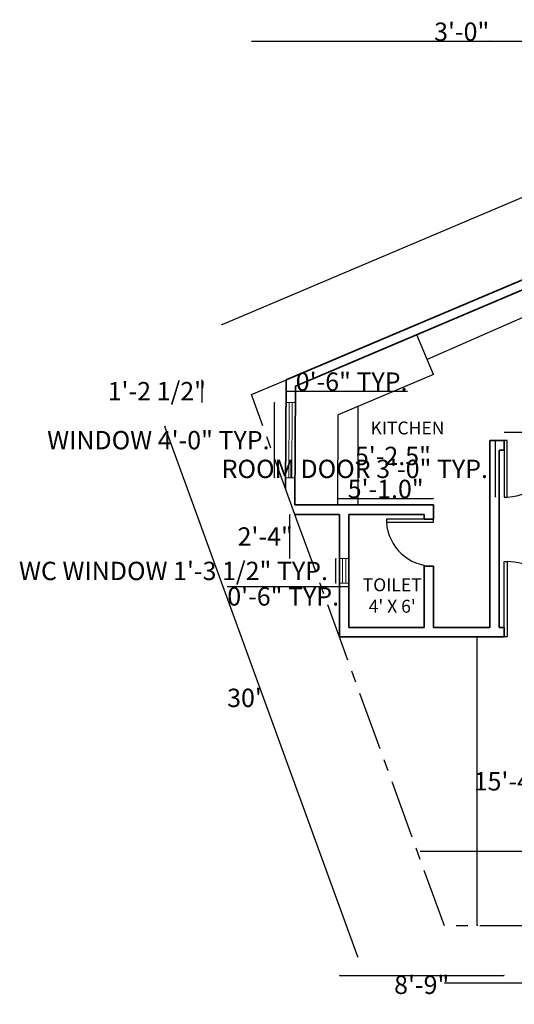
# Model space of a CAD drawing. Units: inches. Extents: x -496 to 183, y 146 to 778.
# Tile 1 of 2: x -496 to -180, y 151 to 778. Entities that reach past the tile are written whole.
import ezdxf

# ---------------------------------------------------------------- set-up
doc = ezdxf.new("R2010")
doc.units = ezdxf.units.IN
doc.header["$MEASUREMENT"] = 0
doc.linetypes.add('CENTER', pattern=[2, 1.25, -0.25, 0.25, -0.25])
for name, color, linetype, lineweight in [('A-ANNO-DIMS', 5, 'Continuous', 18), ('A-AREA-IDEN', 7, 'Continuous', 18), ('A-DOOR', 30, 'Continuous', 25), ('A-FLOR-FIXT', 8, 'Continuous', 25), ('A-GLAZ', 2, 'Continuous', 18), ('A-WALL', 7, 'Continuous', 35), ('C-PROP', 3, 'CENTER', 25)]:
    doc.layers.add(name, color=color, linetype=linetype, lineweight=lineweight)
doc.styles.get("Standard").update_dxf_attribs({"font": 'arial.ttf'})
doc.dimstyles.get("Standard").update_dxf_attribs({"dimtxt": 11.68, "dimasz": 0.18, "dimexe": 0.18, "dimexo": 0.0625, "dimgap": 0.09, "dimtad": 2, "dimtih": 1, "dimtoh": 1, "dimdec": 1, "dimzin": 0, "dimdsep": 46, "dimlunit": 3, "dimtxsty": 'Standard', "dimblk": 'OPEN30', "dimcen": 0.09, "dimse1": 1, "dimse2": 1, "dimadec": 0, "dimazin": 0, "dimtfac": 1, "dimtdec": 1, "dimtofl": 0, "dimtmove": 0, "dimatfit": 3, "dimfxl": 1, "dimtolj": 1, "dimtzin": 0, "dimarcsym": 0})

# ---------------------------------------------------------------- blocks, each defined once
blk = doc.blocks.new('_Open30')
at = {"color": 0, "linetype": 'ByBlock', "lineweight": -2}
for p, q in [((-1, 0.27), (0, 0)), ((0, 0), (-1, -0.27)), ((0, 0), (-1, 0))]:
    blk.add_line(p, q, dxfattribs=at)
blk = doc.blocks.new('*D3')
at = {"layer": 'A-ANNO-DIMS', "color": 0, "lineweight": -2, "ltscale": 5, "transparency": 16777216}
blk.add_line((-224.62, 164.47), (15.02, 164.47), dxfattribs=at)
at = {"layer": 'Defpoints', "color": 0, "ltscale": 5, "transparency": 16777216}
for p in [(-224.8, 200.81), (15.2, 200.81), (15.2, 164.47)]:
    blk.add_point(p, dxfattribs=at)
at = {"layer": 'A-ANNO-DIMS', "color": 0, "lineweight": -2, "ltscale": 5, "transparency": 16777216, "xscale": 0.18, "yscale": 0.18, "zscale": 0.18, "rotation": 180}
blk.add_blockref('_Open30', (-224.8, 164.47), dxfattribs=at)
at = {"layer": 'A-ANNO-DIMS', "color": 0, "lineweight": -2, "ltscale": 5, "transparency": 16777216, "xscale": 0.18, "yscale": 0.18, "zscale": 0.18}
blk.add_blockref('_Open30', (15.2, 164.47), dxfattribs=at)
at = {"layer": 'A-ANNO-DIMS', "color": 0, "ltscale": 5, "transparency": 16777216, "insert": (-104.8, 158.42), "char_height": 11.68, "attachment_point": 5}
blk.add_mtext("\\A1;20'", dxfattribs=at)
blk = doc.blocks.new('*D5')
at = {"layer": 'A-ANNO-DIMS', "color": 0, "lineweight": -2, "ltscale": 5, "transparency": 16777216}
blk.add_line((-280.02, 180.9), (-403.03, 518.85), dxfattribs=at)
at = {"layer": 'Defpoints', "color": 0, "ltscale": 5, "transparency": 16777216}
for p in [(-347.92, 539.1), (-403.09, 519.02), (-224.8, 200.81)]:
    blk.add_point(p, dxfattribs=at)
at = {"layer": 'A-ANNO-DIMS', "color": 0, "lineweight": -2, "ltscale": 5, "transparency": 16777216, "xscale": 0.18, "yscale": 0.18, "zscale": 0.18}
for p, rotation in [((-403.09, 519.02), 109.9999999999999), ((-279.96, 180.73), 290)]:
    blk.add_blockref('_Open30', p, dxfattribs=dict(at, rotation=rotation))
at = {"layer": 'A-ANNO-DIMS', "color": 0, "ltscale": 5, "transparency": 16777216, "insert": (-352.3, 345.96), "char_height": 11.68, "attachment_point": 5}
blk.add_mtext("\\A1;30'", dxfattribs=at)
blk = doc.blocks.new('*D6')
at = {"layer": 'A-ANNO-DIMS', "color": 0, "lineweight": -2, "ltscale": 5, "transparency": 16777216}
blk.add_line((-366.62, 583.72), (89.94, 777.08), dxfattribs=at)
at = {"layer": 'Defpoints', "color": 0, "ltscale": 5, "transparency": 16777216}
for p in [(90.11, 777.15), (108.97, 732.61), (-347.92, 539.1)]:
    blk.add_point(p, dxfattribs=at)
at = {"layer": 'A-ANNO-DIMS', "color": 0, "lineweight": -2, "ltscale": 5, "transparency": 16777216, "xscale": 0.18, "yscale": 0.18, "zscale": 0.18}
for p, rotation in [((90.11, 777.15), 22.95381137769926), ((-366.79, 583.64), 202.9538113776993)]:
    blk.add_blockref('_Open30', p, dxfattribs=dict(at, rotation=rotation))
at = {"layer": 'A-ANNO-DIMS', "color": 0, "ltscale": 5, "transparency": 16777216, "insert": (-144.61, 695.21), "char_height": 11.68, "attachment_point": 5}
blk.add_mtext('\\A1;41\'-4.2"', dxfattribs=at)
blk = doc.blocks.new('*D7')
at = {"layer": 'A-ANNO-DIMS', "color": 0, "lineweight": -2, "ltscale": 5, "transparency": 16777216}
blk.add_line((-235.59, 561.64), (-68.58, 635.31), dxfattribs=at)
at = {"layer": 'Defpoints', "color": 0, "ltscale": 5, "transparency": 16777216}
for p in [(-69.77, 638.45), (-68.41, 635.38), (-237.11, 564.64)]:
    blk.add_point(p, dxfattribs=at)
at = {"layer": 'A-ANNO-DIMS', "color": 0, "lineweight": -2, "ltscale": 5, "transparency": 16777216, "xscale": 0.18, "yscale": 0.18, "zscale": 0.18}
for p, rotation in [((-68.41, 635.38), 23.80147962325558), ((-235.75, 561.57), 203.8014796232556)]:
    blk.add_blockref('_Open30', p, dxfattribs=dict(at, rotation=rotation))
at = {"layer": 'A-ANNO-DIMS', "color": 0, "ltscale": 5, "transparency": 16777216, "insert": (-145.55, 583.66), "char_height": 11.68, "attachment_point": 5}
blk.add_mtext('\\A1;15\'-2.9"', dxfattribs=at)
blk = doc.blocks.new('*D12')
at = {"layer": 'A-ANNO-DIMS', "color": 0, "lineweight": -2, "ltscale": 5, "transparency": 16777216}
blk.add_line((22.65, 248.06), (-240.18, 248.06), dxfattribs=at)
at = {"layer": 'Defpoints', "color": 0, "ltscale": 5, "transparency": 16777216}
for p in [(-240.36, 248.06), (-240.36, 243.58), (22.83, 244.08)]:
    blk.add_point(p, dxfattribs=at)
at = {"layer": 'A-ANNO-DIMS', "color": 0, "lineweight": -2, "ltscale": 5, "transparency": 16777216, "xscale": 0.18, "yscale": 0.18, "zscale": 0.18, "rotation": 180}
blk.add_blockref('_Open30', (-240.36, 248.06), dxfattribs=at)
at = {"layer": 'A-ANNO-DIMS', "color": 0, "lineweight": -2, "ltscale": 5, "transparency": 16777216, "xscale": 0.18, "yscale": 0.18, "zscale": 0.18}
blk.add_blockref('_Open30', (22.83, 248.06), dxfattribs=at)
at = {"layer": 'A-ANNO-DIMS', "color": 0, "ltscale": 5, "transparency": 16777216, "insert": (-108.76, 254.01), "char_height": 11.68, "attachment_point": 5}
blk.add_mtext('\\A1;21\'-11.2"', dxfattribs=at)
blk = doc.blocks.new('*D13')
at = {"layer": 'A-ANNO-DIMS', "color": 0, "lineweight": -2, "ltscale": 5, "transparency": 16777216}
blk.add_line((-203.87, 200.99), (-203.87, 384.63), dxfattribs=at)
at = {"layer": 'Defpoints', "color": 0, "ltscale": 5, "transparency": 16777216}
for p in [(-208.53, 384.81), (-203.87, 384.81), (-208.53, 200.81)]:
    blk.add_point(p, dxfattribs=at)
at = {"layer": 'A-ANNO-DIMS', "color": 0, "lineweight": -2, "ltscale": 5, "transparency": 16777216, "xscale": 0.18, "yscale": 0.18, "zscale": 0.18}
for p, rotation in [((-203.87, 384.81), 90), ((-203.87, 200.81), 270)]:
    blk.add_blockref('_Open30', p, dxfattribs=dict(at, rotation=rotation))
at = {"layer": 'A-ANNO-DIMS', "color": 0, "ltscale": 5, "transparency": 16777216, "insert": (-177.47, 292.81), "char_height": 11.68, "attachment_point": 5}
blk.add_mtext('\\A1;15\'-4.0"', dxfattribs=at)
blk = doc.blocks.new('*D14')
at = {"layer": 'A-ANNO-DIMS', "color": 0, "lineweight": -2, "ltscale": 5, "transparency": 16777216}
blk.add_line((-280.06, 531.08), (-280.06, 468.99), dxfattribs=at)
at = {"layer": 'Defpoints', "color": 0, "ltscale": 5, "transparency": 16777216}
for p in [(-280.79, 531.26), (-280.79, 468.81), (-280.06, 468.81)]:
    blk.add_point(p, dxfattribs=at)
at = {"layer": 'A-ANNO-DIMS', "color": 0, "lineweight": -2, "ltscale": 5, "transparency": 16777216, "xscale": 0.18, "yscale": 0.18, "zscale": 0.18}
for p, rotation in [((-280.06, 531.26), 90), ((-280.06, 468.81), 270)]:
    blk.add_blockref('_Open30', p, dxfattribs=dict(at, rotation=rotation))
at = {"layer": 'A-ANNO-DIMS', "color": 0, "ltscale": 5, "transparency": 16777216, "insert": (-257.64, 500.04), "char_height": 11.68, "attachment_point": 5}
blk.add_mtext('\\A1;5\'-2.5"', dxfattribs=at)
blk = doc.blocks.new('*D15')
at = {"layer": 'A-ANNO-DIMS', "color": 0, "lineweight": -2, "ltscale": 5, "transparency": 16777216}
blk.add_line((-292.55, 472.99), (-231.95, 472.99), dxfattribs=at)
at = {"layer": 'Defpoints', "color": 0, "ltscale": 5, "transparency": 16777216}
for p in [(-231.77, 472.99), (-292.73, 468.81), (-231.77, 468.81)]:
    blk.add_point(p, dxfattribs=at)
at = {"layer": 'A-ANNO-DIMS', "color": 0, "lineweight": -2, "ltscale": 5, "transparency": 16777216, "xscale": 0.18, "yscale": 0.18, "zscale": 0.18, "rotation": 180}
blk.add_blockref('_Open30', (-292.73, 472.99), dxfattribs=at)
at = {"layer": 'A-ANNO-DIMS', "color": 0, "lineweight": -2, "ltscale": 5, "transparency": 16777216, "xscale": 0.18, "yscale": 0.18, "zscale": 0.18}
blk.add_blockref('_Open30', (-231.77, 472.99), dxfattribs=at)
at = {"layer": 'A-ANNO-DIMS', "color": 0, "ltscale": 5, "transparency": 16777216, "insert": (-262.25, 479.04), "char_height": 11.68, "attachment_point": 5}
blk.add_mtext('\\A1;5\'-1.0"', dxfattribs=at)
blk = doc.blocks.new('DOOR-SWING-36IN')
at = {"ltscale": 5}
for p, q in [((0, 0), (0, -36)), ((2, 0), (0, 0)), ((2, -36), (2, 0)), ((0, -36), (2, -36))]:
    blk.add_line(p, q, dxfattribs=at)
blk.add_arc((-0.06, 0), 36.06, 273.27315, 0, dxfattribs=at)
blk = doc.blocks.new('DOOR-SWING-30IN')
at = {"ltscale": 5}
for p, q in [((0, 0), (-30, 0)), ((-30, 0), (-30, -2)), ((0, -2), (0, 0)), ((-30, -2), (0, -2))]:
    blk.add_line(p, q, dxfattribs=at)
blk.add_arc((0, 0.07), 30.07, 183.94987, 270, dxfattribs=at)
blk = doc.blocks.new('WIN-48IN')
at = {"ltscale": 5}
for p, q in [((0, 0), (-0.22, -48)), ((0, 0), (6, -0.03)), ((6, -0.03), (5.78, -48.03)), ((-0.22, -48), (5.78, -48.03))]:
    blk.add_line(p, q, dxfattribs=at)
for p, q in [((1.78, -48.01), (2, -0.01)), ((3.78, -48.02), (4, -0.02))]:
    blk.add_line(p, q)
blk = doc.blocks.new('WIN-SMALL-WC')
at = {"ltscale": 5}
for p, q in [((-15.66, -6), (-15.66, 0)), ((-15.66, 0), (0, 0)), ((0, 0), (0, -6)), ((-15.66, -2), (0, -2)), ((0, -4), (-15.66, -4)), ((0, -6), (-15.66, -6))]:
    blk.add_line(p, q, dxfattribs=at)
blk = doc.blocks.new('*D20')
at = {"layer": 'A-ANNO-DIMS', "color": 0, "lineweight": -2, "ltscale": 5, "transparency": 16777216}
blk.add_line((-192.17, 473.99), (-192.17, 509.63), dxfattribs=at)
at = {"layer": 'Defpoints', "color": 0, "ltscale": 5, "transparency": 16777216}
for p in [(-192.17, 509.81), (-186.77, 509.81), (-186.77, 473.81)]:
    blk.add_point(p, dxfattribs=at)
at = {"layer": 'A-ANNO-DIMS', "color": 0, "lineweight": -2, "ltscale": 5, "transparency": 16777216, "xscale": 0.18, "yscale": 0.18, "zscale": 0.18}
for p, rotation in [((-192.17, 509.81), 90), ((-192.17, 473.81), 270)]:
    blk.add_blockref('_Open30', p, dxfattribs=dict(at, rotation=rotation))
at = {"layer": 'A-ANNO-DIMS', "color": 0, "ltscale": 5, "transparency": 16777216, "insert": (-281.94, 491.81), "char_height": 11.68, "attachment_point": 5}
blk.add_mtext('\\A1;ROOM DOOR 3\'-0" TYP.', dxfattribs=at)
blk = doc.blocks.new('*D21')
at = {"layer": 'A-ANNO-DIMS', "color": 0, "lineweight": -2, "ltscale": 5, "transparency": 16777216}
for p, q in [((-186.59, 515.21), (-150.95, 515.21)), ((-150.77, 515.21), (-79.22, 515.21))]:
    blk.add_line(p, q, dxfattribs=at)
at = {"layer": 'Defpoints', "color": 0, "ltscale": 5, "transparency": 16777216}
for p in [(-150.77, 515.21), (-186.77, 509.81), (-150.77, 509.81)]:
    blk.add_point(p, dxfattribs=at)
at = {"layer": 'A-ANNO-DIMS', "color": 0, "lineweight": -2, "ltscale": 5, "transparency": 16777216, "xscale": 0.18, "yscale": 0.18, "zscale": 0.18, "rotation": 180}
blk.add_blockref('_Open30', (-186.77, 515.21), dxfattribs=at)
at = {"layer": 'A-ANNO-DIMS', "color": 0, "lineweight": -2, "ltscale": 5, "transparency": 16777216, "xscale": 0.18, "yscale": 0.18, "zscale": 0.18}
blk.add_blockref('_Open30', (-150.77, 515.21), dxfattribs=at)
at = {"layer": 'A-ANNO-DIMS', "color": 0, "ltscale": 5, "transparency": 16777216, "insert": (-114.9, 521.27), "char_height": 11.68, "attachment_point": 5}
blk.add_mtext('\\A1;3\'-0" TYP.', dxfattribs=at)
blk = doc.blocks.new('*D24')
at = {"layer": 'A-ANNO-DIMS', "color": 0, "lineweight": -2, "ltscale": 5, "transparency": 16777216}
blk.add_line((-333.25, 486.28), (-333.25, 533.95), dxfattribs=at)
at = {"layer": 'Defpoints', "color": 0, "ltscale": 5, "transparency": 16777216}
for p in [(-333.25, 534.13), (-326.05, 534.13), (-326.05, 486.1)]:
    blk.add_point(p, dxfattribs=at)
at = {"layer": 'A-ANNO-DIMS', "color": 0, "lineweight": -2, "ltscale": 5, "transparency": 16777216, "xscale": 0.18, "yscale": 0.18, "zscale": 0.18}
for p, rotation in [((-333.25, 534.13), 90), ((-333.25, 486.1), 270)]:
    blk.add_blockref('_Open30', p, dxfattribs=dict(at, rotation=rotation))
at = {"layer": 'A-ANNO-DIMS', "color": 0, "ltscale": 5, "transparency": 16777216, "insert": (-407.24, 510.11), "char_height": 11.68, "attachment_point": 5}
blk.add_mtext('\\A1;WINDOW 4\'-0" TYP.', dxfattribs=at)
blk = doc.blocks.new('*D25')
at = {"layer": 'A-ANNO-DIMS', "color": 0, "lineweight": -2, "ltscale": 5, "transparency": 16777216}
for p, q in [((-325.87, 541.33), (-320.01, 541.33)), ((-319.83, 541.33), (-248.28, 541.33))]:
    blk.add_line(p, q, dxfattribs=at)
at = {"layer": 'Defpoints', "color": 0, "ltscale": 5, "transparency": 16777216}
for p in [(-319.83, 541.33), (-326.05, 534.13), (-319.83, 534.13)]:
    blk.add_point(p, dxfattribs=at)
at = {"layer": 'A-ANNO-DIMS', "color": 0, "lineweight": -2, "ltscale": 5, "transparency": 16777216, "xscale": 0.18, "yscale": 0.18, "zscale": 0.18, "rotation": 180}
blk.add_blockref('_Open30', (-326.05, 541.33), dxfattribs=at)
at = {"layer": 'A-ANNO-DIMS', "color": 0, "lineweight": -2, "ltscale": 5, "transparency": 16777216, "xscale": 0.18, "yscale": 0.18, "zscale": 0.18}
blk.add_blockref('_Open30', (-319.83, 541.33), dxfattribs=at)
at = {"layer": 'A-ANNO-DIMS', "color": 0, "ltscale": 5, "transparency": 16777216, "insert": (-283.97, 547.38), "char_height": 11.68, "attachment_point": 5}
blk.add_mtext('\\A1;0\'-6" TYP.', dxfattribs=at)
blk = doc.blocks.new('*D26')
at = {"layer": 'A-ANNO-DIMS', "color": 0, "lineweight": -2, "ltscale": 5, "transparency": 16777216}
blk.add_line((-294.11, 419.16), (-294.11, 434.46), dxfattribs=at)
at = {"layer": 'Defpoints', "color": 0, "ltscale": 5, "transparency": 16777216}
for p in [(-294.11, 434.64), (-291.77, 434.64), (-291.77, 418.98)]:
    blk.add_point(p, dxfattribs=at)
at = {"layer": 'A-ANNO-DIMS', "color": 0, "lineweight": -2, "ltscale": 5, "transparency": 16777216, "xscale": 0.18, "yscale": 0.18, "zscale": 0.18}
for p, rotation in [((-294.11, 434.64), 90), ((-294.11, 418.98), 270)]:
    blk.add_blockref('_Open30', p, dxfattribs=dict(at, rotation=rotation))
at = {"layer": 'A-ANNO-DIMS', "color": 0, "ltscale": 5, "transparency": 16777216, "insert": (-397.57, 426.81), "char_height": 11.68, "attachment_point": 5}
blk.add_mtext('\\A1;WC WINDOW 1\'-3 1/2" TYP.', dxfattribs=at)
blk = doc.blocks.new('*D27')
at = {"layer": 'A-ANNO-DIMS', "color": 0, "lineweight": -2, "ltscale": 5, "transparency": 16777216}
for p, q in [((-291.77, 416.64), (-363.32, 416.64)), ((-285.95, 416.64), (-291.59, 416.64))]:
    blk.add_line(p, q, dxfattribs=at)
at = {"layer": 'Defpoints', "color": 0, "ltscale": 5, "transparency": 16777216}
for p in [(-291.77, 418.98), (-291.77, 416.64), (-285.77, 418.98)]:
    blk.add_point(p, dxfattribs=at)
at = {"layer": 'A-ANNO-DIMS', "color": 0, "lineweight": -2, "ltscale": 5, "transparency": 16777216, "xscale": 0.18, "yscale": 0.18, "zscale": 0.18}
for p, rotation in [((-291.77, 416.64), 179.9999999999984), ((-285.77, 416.64), 359.9999999999984)]:
    blk.add_blockref('_Open30', p, dxfattribs=dict(at, rotation=rotation))
at = {"layer": 'A-ANNO-DIMS', "color": 0, "ltscale": 5, "transparency": 16777216, "insert": (-327.63, 410.58), "char_height": 11.68, "attachment_point": 5}
blk.add_mtext('\\A1;0\'-6" TYP.', dxfattribs=at)
blk = doc.blocks.new('*D28')
at = {"layer": 'A-ANNO-DIMS', "color": 0, "lineweight": -2, "ltscale": 5, "transparency": 16777216}
blk.add_line((-347.74, 764.21), (108.79, 764.21), dxfattribs=at)
at = {"layer": 'Defpoints', "color": 0, "ltscale": 5, "transparency": 16777216}
for p in [(108.97, 764.21), (108.97, 732.61), (-347.92, 539.1)]:
    blk.add_point(p, dxfattribs=at)
at = {"layer": 'A-ANNO-DIMS', "color": 0, "lineweight": -2, "ltscale": 5, "transparency": 16777216, "xscale": 0.18, "yscale": 0.18, "zscale": 0.18, "rotation": 180}
blk.add_blockref('_Open30', (-347.92, 764.21), dxfattribs=at)
at = {"layer": 'A-ANNO-DIMS', "color": 0, "lineweight": -2, "ltscale": 5, "transparency": 16777216, "xscale": 0.18, "yscale": 0.18, "zscale": 0.18}
blk.add_blockref('_Open30', (108.97, 764.21), dxfattribs=at)
at = {"layer": 'A-ANNO-DIMS', "color": 0, "ltscale": 5, "transparency": 16777216, "insert": (-119.47, 770.27), "char_height": 11.68, "attachment_point": 5}
blk.add_mtext('\\A1;38\'-1"', dxfattribs=at)
blk = doc.blocks.new('*D31')
at = {"layer": 'A-ANNO-DIMS', "color": 0, "lineweight": -2, "ltscale": 5, "transparency": 16777216}
blk.add_line((-231.59, 764.21), (-195.95, 764.21), dxfattribs=at)
at = {"layer": 'Defpoints', "color": 0, "ltscale": 5, "transparency": 16777216}
for p in [(-195.77, 764.21), (-231.77, 390.81), (-195.77, 390.81)]:
    blk.add_point(p, dxfattribs=at)
at = {"layer": 'A-ANNO-DIMS', "color": 0, "lineweight": -2, "ltscale": 5, "transparency": 16777216, "xscale": 0.18, "yscale": 0.18, "zscale": 0.18, "rotation": 180}
blk.add_blockref('_Open30', (-231.77, 764.21), dxfattribs=at)
at = {"layer": 'A-ANNO-DIMS', "color": 0, "lineweight": -2, "ltscale": 5, "transparency": 16777216, "xscale": 0.18, "yscale": 0.18, "zscale": 0.18}
blk.add_blockref('_Open30', (-195.77, 764.21), dxfattribs=at)
at = {"layer": 'A-ANNO-DIMS', "color": 0, "ltscale": 5, "transparency": 16777216, "insert": (-213.77, 770.27), "char_height": 11.68, "attachment_point": 5}
blk.add_mtext('\\A1;3\'-0"', dxfattribs=at)
blk = doc.blocks.new('*D32')
at = {"layer": 'A-ANNO-DIMS', "color": 0, "lineweight": -2, "ltscale": 5, "transparency": 16777216}
blk.add_line((-291.59, 169.21), (-186.95, 169.21), dxfattribs=at)
at = {"layer": 'Defpoints', "color": 0, "ltscale": 5, "transparency": 16777216}
for p in [(-291.77, 384.81), (-186.77, 384.81), (-186.77, 169.21)]:
    blk.add_point(p, dxfattribs=at)
at = {"layer": 'A-ANNO-DIMS', "color": 0, "lineweight": -2, "ltscale": 5, "transparency": 16777216, "xscale": 0.18, "yscale": 0.18, "zscale": 0.18, "rotation": 180}
blk.add_blockref('_Open30', (-291.77, 169.21), dxfattribs=at)
at = {"layer": 'A-ANNO-DIMS', "color": 0, "lineweight": -2, "ltscale": 5, "transparency": 16777216, "xscale": 0.18, "yscale": 0.18, "zscale": 0.18}
blk.add_blockref('_Open30', (-186.77, 169.21), dxfattribs=at)
at = {"layer": 'A-ANNO-DIMS', "color": 0, "ltscale": 5, "transparency": 16777216, "insert": (-239.27, 163.16), "char_height": 11.68, "attachment_point": 5}
blk.add_mtext('\\A1;8\'-9"', dxfattribs=at)
blk = doc.blocks.new('*D35')
at = {"layer": 'A-ANNO-DIMS', "color": 0, "lineweight": -2, "ltscale": 5, "transparency": 16777216}
blk.add_line((-379.52, 548.3), (-379.52, 534.31), dxfattribs=at)
at = {"layer": 'Defpoints', "color": 0, "ltscale": 5, "transparency": 16777216}
for p in [(-325.77, 548.48), (-379.52, 534.13), (-325.83, 534.13)]:
    blk.add_point(p, dxfattribs=at)
at = {"layer": 'A-ANNO-DIMS', "color": 0, "lineweight": -2, "ltscale": 5, "transparency": 16777216, "xscale": 0.18, "yscale": 0.18, "zscale": 0.18}
for p, rotation in [((-379.52, 548.48), 90), ((-379.52, 534.13), 270)]:
    blk.add_blockref('_Open30', p, dxfattribs=dict(at, rotation=rotation))
at = {"layer": 'A-ANNO-DIMS', "color": 0, "ltscale": 5, "transparency": 16777216, "insert": (-408.2, 541.3), "char_height": 11.68, "attachment_point": 5}
blk.add_mtext('\\A1;1\'-2 1/2"', dxfattribs=at)
blk = doc.blocks.new('*D39')
at = {"layer": 'A-ANNO-DIMS', "color": 0, "lineweight": -2, "ltscale": 5, "transparency": 16777216}
blk.add_line((-323.37, 434.82), (-323.37, 462.63), dxfattribs=at)
at = {"layer": 'Defpoints', "color": 0, "ltscale": 5, "transparency": 16777216}
for p in [(-323.37, 462.81), (-291.77, 462.81), (-291.77, 434.64)]:
    blk.add_point(p, dxfattribs=at)
at = {"layer": 'A-ANNO-DIMS', "color": 0, "lineweight": -2, "ltscale": 5, "transparency": 16777216, "xscale": 0.18, "yscale": 0.18, "zscale": 0.18}
for p, rotation in [((-323.37, 462.81), 90), ((-323.37, 434.64), 270)]:
    blk.add_blockref('_Open30', p, dxfattribs=dict(at, rotation=rotation))
at = {"layer": 'A-ANNO-DIMS', "color": 0, "ltscale": 5, "transparency": 16777216, "insert": (-339.08, 448.73), "char_height": 11.68, "attachment_point": 5}
blk.add_mtext('\\A1;2\'-4"', dxfattribs=at)
blk = doc.blocks.new('*D40')
at = {"layer": 'A-ANNO-DIMS', "color": 0, "lineweight": -2, "ltscale": 5, "transparency": 16777216}
for p, q in [((-131.31, 438), (-151.99, 418.18)), ((-88.99, 438), (-131.31, 438)), ((-186.9, 384.81), (-186.72, 384.81)), ((-186.81, 384.72), (-186.81, 384.9))]:
    blk.add_line(p, q, dxfattribs=at)
at = {"layer": 'Defpoints', "color": 0, "ltscale": 5, "transparency": 16777216}
for p in [(-152.12, 418.05), (-186.81, 384.81)]:
    blk.add_point(p, dxfattribs=at)
at = {"layer": 'A-ANNO-DIMS', "color": 0, "lineweight": -2, "ltscale": 5, "transparency": 16777216, "xscale": 0.18, "yscale": 0.18, "zscale": 0.18, "rotation": 223.7807826130634}
blk.add_blockref('_Open30', (-152.12, 418.05), dxfattribs=at)
at = {"layer": 'A-ANNO-DIMS', "color": 0, "ltscale": 5, "transparency": 16777216, "insert": (-110.11, 444.05), "char_height": 11.68, "attachment_point": 5}
blk.add_mtext('\\A1;R4\'-0"', dxfattribs=at)

msp = doc.modelspace()

# ---------------------------------------------------------------- linework, layer by layer
at = {"layer": 'A-DOOR', "ltscale": 5}
for p, q in [((-186.77, 384.81), (-186.77, 432.81)), ((-186.77, 432.81), (-184.77, 432.81)), ((-184.77, 432.81), (-184.77, 384.81)), ((-184.77, 384.81), (-186.77, 384.81))]:
    msp.add_line(p, q, dxfattribs=at)
msp.add_arc((-186.81, 384.81), 48.04, 0, 87.56225, dxfattribs=at)
at = {"layer": 'A-FLOR-FIXT'}
for p, q in [((-231.77, 552.02), (-242.45, 577.26)), ((-231.77, 552.02), (-292.47, 526.32)), ((-292.73, 468.69), (-292.47, 526.32))]:
    msp.add_line(p, q, dxfattribs=at)
at = {"layer": 'A-WALL', "ltscale": 5}
msp.add_line((-64.98, 658.93), (-325.77, 548.48), dxfattribs=at)
at = {"layer": 'A-WALL'}
for p, q in [((-69.77, 650.39), (-319.79, 544.5)), ((-326.08, 479.1), (-325.77, 548.48)), ((-320.13, 468.81), (-319.79, 544.5)), ((-195.77, 509.81), (-186.77, 509.81)), ((-195.77, 390.81), (-195.77, 509.81)), ((-186.77, 503.81), (-186.77, 509.81)), ((-189.77, 503.81), (-186.77, 503.81)), ((-189.77, 390.81), (-189.77, 503.81)), ((-320.13, 468.81), (-231.77, 468.81)), ((-231.77, 459.81), (-231.77, 468.81)), ((-320.16, 462.81), (-291.77, 462.81)), ((-291.77, 384.81), (-291.77, 462.81)), ((-285.77, 390.81), (-285.77, 462.81)), ((-285.77, 462.81), (-237.77, 462.81)), ((-237.77, 459.81), (-237.77, 462.81)), ((-237.77, 459.81), (-231.77, 459.81)), ((-237.77, 390.81), (-237.77, 429.81)), ((-237.77, 429.81), (-231.77, 429.81)), ((-231.77, 390.81), (-231.77, 429.81)), ((-285.77, 390.81), (-237.77, 390.81)), ((-231.77, 390.81), (-195.77, 390.81)), ((-189.77, 390.81), (-186.77, 390.81)), ((-186.77, 384.81), (-186.77, 390.81)), ((-291.77, 384.81), (-186.77, 384.81))]:
    msp.add_line(p, q, dxfattribs=at)
at = {"layer": 'C-PROP', "ltscale": 30}
msp.add_lwpolyline([(-320.16, 462.81), (-347.92, 539.1), (108.97, 732.61), (15.2, 200.81), (-224.8, 200.81), (-319.06, 459.81)], close=True, dxfattribs=at)

# ---------------------------------------------------------------- block references
at = {"layer": 'A-DOOR'}
for name, p in [('DOOR-SWING-36IN', (-186.77, 509.81)), ('DOOR-SWING-30IN', (-231.77, 459.81))]:
    msp.add_blockref(name, p, dxfattribs=at)
at = {"layer": 'A-GLAZ'}
msp.add_blockref('WIN-48IN', (-325.83, 534.13), dxfattribs=at)
at = {"layer": 'A-GLAZ', "rotation": 89.9999999999982}
msp.add_blockref('WIN-SMALL-WC', (-291.77, 434.64), dxfattribs=at)

# ---------------------------------------------------------------- texts
at = {"layer": 'A-AREA-IDEN', "ltscale": 5, "char_height": 8.2, "attachment_point": 1}
for s, width, insert in [('KITCHEN', 1.3024, (-271.95, 521.96)), ("\\pxqc;TOILET\\P4' X 6'", 37.7679, (-276.97, 422.07))]:
    msp.add_mtext_dynamic_manual_height_columns(s, width=width, gutter_width=1, heights=[0], dxfattribs=dict(at, insert=insert))

# ---------------------------------------------------------------- dimensions: what is measured, and where the dimension line sits
at = {"layer": 'A-ANNO-DIMS', "ltscale": 5}
for base, p1, p2, override, picture, middle in [((108.97, 764.21), (-347.92, 539.1), (108.97, 732.61), {"dimdec": 1, "dimlfac": 1, "dimrnd": 0, "dimzin": 1, "dimdsep": 46, "dimlunit": 4, "dimfrac": 2}, '*D28', (-119.47, 770.27)), ((-195.77, 764.21), (-231.77, 390.81), (-195.77, 390.81), {"dimdec": 1, "dimlfac": 1, "dimrnd": 0, "dimzin": 1, "dimdsep": 46, "dimlunit": 4, "dimfrac": 2}, '*D31', (-213.77, 770.27)), ((-231.77, 472.99), (-292.73, 468.81), (-231.77, 468.81), {"dimclrd": 0, "dimclre": 0, "dimclrt": 0}, '*D15', (-262.25, 479.04)), ((-186.77, 169.21), (-291.77, 384.81), (-186.77, 384.81), {"dimdec": 1, "dimlfac": 1, "dimrnd": 0, "dimzin": 1, "dimdsep": 46, "dimlunit": 4, "dimfrac": 2}, '*D32', (-239.27, 163.16)), ((-240.36, 248.06), (22.83, 244.08), (-240.36, 243.58), {"dimclrd": 0, "dimclre": 0, "dimclrt": 0}, '*D12', (-108.76, 254.01)), ((15.2, 164.47), (-224.8, 200.81), (15.2, 200.81), {"dimclrd": 0, "dimclre": 0, "dimclrt": 0}, '*D3', (-104.8, 158.42))]:
    dim = msp.add_linear_dim(base=base, p1=p1, p2=p2, dimstyle='Standard', override=override, dxfattribs=at)
    dim.commit()
    dim.dimension.update_dxf_attribs({"geometry": picture, "text_midpoint": middle})
for p1, p2, distance, picture, middle in [((-347.92, 539.1), (108.97, 732.61), 48.37, '*D6', (-144.61, 695.21)), ((-237.11, 564.64), (-69.77, 638.45), -3.35, '*D7', (-145.55, 583.66)), ((-224.8, 200.81), (-347.92, 539.1), 58.71, '*D5', (-352.3, 345.96))]:
    dim = msp.add_aligned_dim(p1=p1, p2=p2, distance=distance, dimstyle='Standard', override={"dimclrd": 0, "dimclre": 0, "dimclrt": 0}, dxfattribs=at)
    dim.commit()
    dim.dimension.update_dxf_attribs({"geometry": picture, "text_midpoint": middle})
for base, p1, p2, picture, middle in [((-319.83, 541.33), (-326.05, 534.13), (-319.83, 534.13), '*D25', (-283.97, 547.38)), ((-150.77, 515.21), (-186.77, 509.81), (-150.77, 509.81), '*D21', (-114.9, 521.27))]:
    dim = msp.add_linear_dim(base=base, p1=p1, p2=p2, text='<> TYP.', dimstyle='Standard', override={"dimdec": 1, "dimlfac": 1, "dimrnd": 0, "dimzin": 1, "dimdsep": 46, "dimlunit": 4, "dimfrac": 2}, dxfattribs=at)
    dim.commit()
    dim.dimension.update_dxf_attribs({"geometry": picture, "text_midpoint": middle})
for base, p1, p2, override, picture, middle in [((-379.5226, 534.1252), (-325.7703, 548.4838), (-325.8349, 534.1252), {"dimdec": 1, "dimlfac": 1, "dimrnd": 0, "dimzin": 1, "dimdsep": 46, "dimlunit": 4, "dimfrac": 2}, '*D35', (-408.1951, 541.3045)), ((-280.055, 468.8124), (-280.7869, 531.2632), (-280.7869, 468.8124), {"dimclrd": 0, "dimclre": 0, "dimclrt": 0}, '*D14', (-257.6368, 500.0378)), ((-323.37, 462.81), (-291.77, 434.64), (-291.77, 462.81), {"dimdec": 1, "dimlfac": 1, "dimrnd": 0, "dimzin": 1, "dimdsep": 46, "dimlunit": 4, "dimfrac": 2}, '*D39', (-339.08, 448.73)), ((-203.87, 384.81), (-208.53, 200.81), (-208.53, 384.81), {"dimclrd": 0, "dimclre": 0, "dimclrt": 0}, '*D13', (-177.47, 292.81))]:
    dim = msp.add_linear_dim(base=base, p1=p1, p2=p2, angle=90, dimstyle='Standard', override=override, dxfattribs=at)
    dim.commit()
    dim.dimension.update_dxf_attribs({"geometry": picture, "text_midpoint": middle})
for base, p1, p2, angle, text, picture, middle in [((-333.25, 534.13), (-326.05, 486.1), (-326.05, 534.13), 90, 'WINDOW <> TYP.', '*D24', (-407.24, 510.11)), ((-192.17, 509.81), (-186.77, 473.81), (-186.77, 509.81), 90, 'ROOM DOOR <> TYP.', '*D20', (-281.94, 491.81)), ((-294.11, 434.64), (-291.77, 418.98), (-291.77, 434.64), 90, 'WC WINDOW <> TYP.', '*D26', (-397.57, 426.81)), ((-291.77, 416.64), (-285.77, 418.98), (-291.77, 418.98), 180, '<> TYP.', '*D27', (-327.63, 410.58))]:
    dim = msp.add_linear_dim(base=base, p1=p1, p2=p2, angle=angle, text=text, dimstyle='Standard', override={"dimdec": 1, "dimlfac": 1, "dimrnd": 0, "dimzin": 1, "dimdsep": 46, "dimlunit": 4, "dimfrac": 2}, dxfattribs=at)
    dim.commit()
    dim.dimension.update_dxf_attribs({"geometry": picture, "text_midpoint": middle})
dim = msp.add_radius_dim(center=(-186.81, 384.81), mpoint=(-152.12, 418.05), dimstyle='Standard', override={"dimdec": 1, "dimlfac": 1, "dimrnd": 0, "dimzin": 1, "dimdsep": 46, "dimlunit": 4, "dimfrac": 2}, dxfattribs=at)
dim.commit()
dim.dimension.update_dxf_attribs({"geometry": '*D40', "text_midpoint": (-110.11, 438), "dimtype": 164})

doc.saveas('drawing.dxf')
